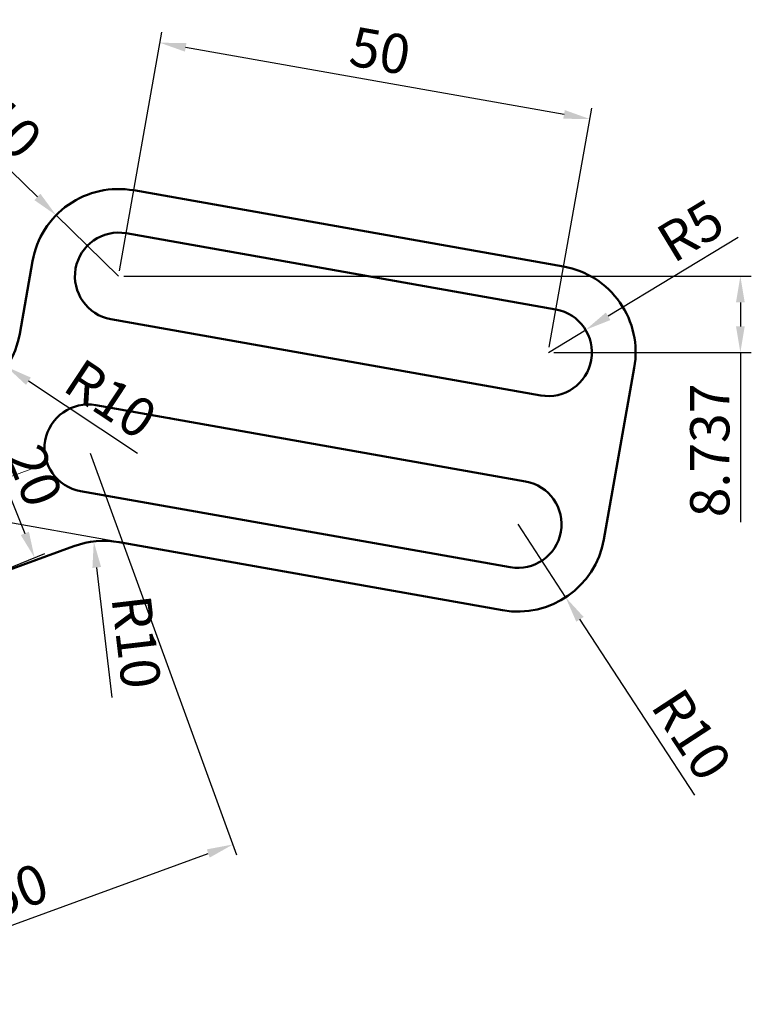
# Model space of a CAD drawing. Units: millimetres. Extents: x 54 to 254, y 16 to 193.
# Tile 2 of 2: x 170 to 254, y 27 to 140. Entities that reach past the tile are written whole.
import ezdxf

# ---------------------------------------------------------------- set-up
doc = ezdxf.new("R2010")
doc.units = ezdxf.units.MM
doc.linetypes.add('CENTER', pattern=[50.8, 31.75, -6.35, 6.35, -6.35])
for name, color, linetype, lineweight in [('M-CNTR', 1, 'CENTER', 18), ('M-DIMS', 2, 'Continuous', 25), ('M-OUTL', 7, 'Continuous', 50)]:
    doc.layers.add(name, color=color, linetype=linetype, lineweight=lineweight)
doc.styles.get("Standard").update_dxf_attribs({"font": 'arial.ttf'})
doc.dimstyles.new('ISO-25', dxfattribs={"dimtxt": 4.5, "dimasz": 3, "dimexe": 1.25, "dimexo": 0.625, "dimtad": 1, "dimdec": 0, "dimtxsty": 'Standard', "dimcen": 2.5, "dimadec": 0, "dimazin": 0, "dimtfac": 1, "dimtdec": 0, "dimtmove": 0, "dimatfit": 3, "dimfxl": 1, "dimarcsym": 0})

# ---------------------------------------------------------------- blocks, each defined once
blk = doc.blocks.new('*D2')
at = {"layer": 'Defpoints', "color": 0, "transparency": 16777216}
for p in [(186.4, 137.25), (181.65, 110.49), (230.91, 101.75)]:
    blk.add_point(p, dxfattribs=at)
at = {"layer": 'M-DIMS', "color": 0, "lineweight": -2, "transparency": 16777216}
for p, q in [((181.76, 111.11), (186.62, 138.48)), ((232.7, 129.04), (189.35, 136.72)), ((231.01, 102.37), (235.87, 129.74))]:
    blk.add_line(p, q, dxfattribs=at)
at = {"layer": 'M-DIMS', "color": 0, "transparency": 16777216}
for points in [[(189.44, 137.22), (189.27, 136.23), (186.4, 137.25)], [(232.79, 129.53), (232.61, 128.54), (235.65, 128.51)]]:
    blk.add_solid(points, dxfattribs=at)
at = {"layer": 'M-DIMS', "color": 0, "transparency": 16777216, "insert": (211.54, 135.76), "char_height": 4.5, "attachment_point": 5, "rotation": 349.9405}
blk.add_mtext('50', dxfattribs=at)
blk = doc.blocks.new('*D20')
at = {"layer": 'Defpoints', "color": 0, "transparency": 16777216}
for p in [(155.74, 93.25), (172.04, 78.24), (163.21, 74.69)]:
    blk.add_point(p, dxfattribs=at)
at = {"layer": 'M-DIMS', "color": 0, "lineweight": -2, "transparency": 16777216}
for p, q in [((156.32, 93.48), (165.74, 97.27)), ((165.7, 94.02), (170.92, 81.02)), ((163.79, 74.92), (173.2, 78.7))]:
    blk.add_line(p, q, dxfattribs=at)
at = {"layer": 'M-DIMS', "color": 0, "transparency": 16777216}
for points in [[(166.16, 94.21), (165.23, 93.83), (164.58, 96.8)], [(171.39, 81.21), (170.46, 80.83), (172.04, 78.24)]]:
    blk.add_solid(points, dxfattribs=at)
at = {"layer": 'M-DIMS', "color": 0, "transparency": 16777216, "insert": (171.5, 87.42), "char_height": 4.5, "attachment_point": 5, "rotation": 291.9033}
blk.add_mtext('20', dxfattribs=at)
blk = doc.blocks.new('*D23')
at = {"layer": 'Defpoints', "color": 0, "transparency": 16777216}
for p in [(178.82, 80.09), (179.98, 70.16)]:
    blk.add_point(p, dxfattribs=at)
at = {"layer": 'M-DIMS', "color": 0, "lineweight": -2, "transparency": 16777216}
blk.add_line((180.92, 62.23), (179.17, 77.11), dxfattribs=at)
at = {"layer": 'M-DIMS', "color": 0, "transparency": 16777216}
blk.add_solid([(179.66, 77.17), (178.67, 77.06), (178.82, 80.09)], dxfattribs=at)
at = {"layer": 'M-DIMS', "color": 0, "transparency": 16777216, "insert": (183.12, 68.52), "char_height": 4.5, "attachment_point": 5, "rotation": 276.7092}
blk.add_mtext('R10', dxfattribs=at)
blk = doc.blocks.new('*D24')
at = {"layer": 'Defpoints', "color": 0, "transparency": 16777216}
for p in [(178.18, 90.79), (131.21, 73.65), (194.76, 45.37)]:
    blk.add_point(p, dxfattribs=at)
at = {"layer": 'M-DIMS', "color": 0, "lineweight": -2, "transparency": 16777216}
for p, q in [((178.4, 90.21), (195.19, 44.19)), ((131.42, 73.07), (148.22, 27.05)), ((150.61, 29.26), (191.94, 44.34))]:
    blk.add_line(p, q, dxfattribs=at)
at = {"layer": 'M-DIMS', "color": 0, "transparency": 16777216}
for points in [[(191.77, 44.81), (192.11, 43.87), (194.76, 45.37)], [(150.43, 29.73), (150.78, 28.79), (147.79, 28.23)]]:
    blk.add_solid(points, dxfattribs=at)
at = {"layer": 'M-DIMS', "color": 0, "transparency": 16777216, "insert": (170.27, 39.54), "char_height": 4.5, "attachment_point": 5, "rotation": 20.0485}
blk.add_mtext('50', dxfattribs=at)
blk = doc.blocks.new('*D25')
at = {"layer": 'Defpoints', "color": 0, "transparency": 16777216}
for p in [(227.41, 82.06), (232.88, 73.69)]:
    blk.add_point(p, dxfattribs=at)
at = {"layer": 'M-DIMS', "color": 0, "lineweight": -2, "transparency": 16777216}
for p, q in [((227.41, 82.06), (232.88, 73.69)), ((247.67, 51.04), (234.52, 71.18))]:
    blk.add_line(p, q, dxfattribs=at)
at = {"layer": 'M-DIMS', "color": 0, "transparency": 16777216}
blk.add_solid([(234.94, 71.45), (234.1, 70.9), (232.88, 73.69)], dxfattribs=at)
at = {"layer": 'M-DIMS', "color": 0, "transparency": 16777216, "insert": (246.84, 57.65), "char_height": 4.5, "attachment_point": 5, "rotation": 303.1406}
blk.add_mtext('R10', dxfattribs=at)
blk = doc.blocks.new('*D26')
at = {"layer": 'Defpoints', "color": 0, "transparency": 16777216}
for p in [(235.18, 104.35), (230.91, 101.75)]:
    blk.add_point(p, dxfattribs=at)
at = {"layer": 'M-DIMS', "color": 0, "lineweight": -2, "transparency": 16777216}
for p, q in [((252.65, 114.94), (237.75, 105.9)), ((230.91, 101.75), (235.18, 104.35))]:
    blk.add_line(p, q, dxfattribs=at)
at = {"layer": 'M-DIMS', "color": 0, "transparency": 16777216}
blk.add_solid([(237.49, 106.33), (238.01, 105.47), (235.18, 104.35)], dxfattribs=at)
at = {"layer": 'M-DIMS', "color": 0, "transparency": 16777216, "insert": (247.49, 115.22), "char_height": 4.5, "attachment_point": 5, "rotation": 31.2309}
blk.add_mtext('R5', dxfattribs=at)
blk = doc.blocks.new('*D27')
at = {"layer": 'Defpoints', "color": 0, "transparency": 16777216}
for p in [(178.18, 90.79), (181.73, 80.01), (156.21, 75.03), (131.21, 73.65), (225.67, 72.21)]:
    blk.add_point(p, dxfattribs=at)
at = {"layer": 'M-DIMS', "color": 0, "lineweight": -2, "transparency": 16777216}
blk.add_line((181.12, 80.12), (167.58, 82.52), dxfattribs=at)
blk.add_arc((159.45, 83.96), 9.5, 218.2164, 331.7726, dxfattribs=at)
at = {"layer": 'M-DIMS', "color": 0, "transparency": 16777216}
for points in [[(167.35, 79.63), (168.3, 79.3), (168.81, 82.3)], [(151.55, 77.84), (152.43, 78.33), (150.53, 80.7)]]:
    blk.add_solid(points, dxfattribs=at)
at = {"layer": 'M-DIMS', "color": 0, "transparency": 16777216, "insert": (160.03, 77.41), "char_height": 4.5, "attachment_point": 5, "rotation": 4.9945}
blk.add_mtext('150°', dxfattribs=at)
blk = doc.blocks.new('SLOT-50X10')
for p, q in [((5.87, 18.66), (55.1, 9.92)), ((4.13, 8.81), (53.36, 0.08))]:
    blk.add_line(p, q)
for centre, start, end in [((5, 13.73), 79.9405, 259.9405), ((54.23, 5), 259.9405, 79.9405)]:
    blk.add_arc(centre, 5, start, end)
blk = doc.blocks.new('*D32')
at = {"layer": 'Defpoints', "color": 0, "transparency": 16777216}
for p in [(181.65, 110.49), (230.91, 101.75), (252.9, 101.75)]:
    blk.add_point(p, dxfattribs=at)
at = {"layer": 'M-DIMS', "color": 0, "lineweight": -2, "transparency": 16777216}
for p, q in [((182.28, 110.49), (254.15, 110.49)), ((252.9, 107.49), (252.9, 104.75)), ((231.53, 101.75), (254.15, 101.75)), ((252.9, 101.75), (252.9, 82.31))]:
    blk.add_line(p, q, dxfattribs=at)
at = {"layer": 'M-DIMS', "color": 0, "transparency": 16777216}
for points in [[(252.4, 107.49), (253.4, 107.49), (252.9, 110.49)], [(252.4, 104.75), (253.4, 104.75), (252.9, 101.75)]]:
    blk.add_solid(points, dxfattribs=at)
at = {"layer": 'M-DIMS', "color": 0, "transparency": 16777216, "insert": (249.98, 90.53), "char_height": 4.5, "attachment_point": 5, "rotation": 90}
blk.add_mtext('8.737', dxfattribs=at)
blk = doc.blocks.new('*D41')
at = {"layer": 'Defpoints', "color": 0, "transparency": 16777216}
for p in [(160.49, 105.63), (168.83, 100.11)]:
    blk.add_point(p, dxfattribs=at)
at = {"layer": 'M-DIMS', "color": 0, "lineweight": -2, "transparency": 16777216}
for p, q in [((160.49, 105.63), (168.83, 100.11)), ((183.83, 90.19), (171.33, 98.46))]:
    blk.add_line(p, q, dxfattribs=at)
at = {"layer": 'M-DIMS', "color": 0, "transparency": 16777216}
blk.add_solid([(171.61, 98.88), (171.06, 98.04), (168.83, 100.11)], dxfattribs=at)
at = {"layer": 'M-DIMS', "color": 0, "transparency": 16777216, "insert": (180.45, 95.94), "char_height": 4.5, "attachment_point": 5, "rotation": 326.5309}
blk.add_mtext('R10', dxfattribs=at)
blk = doc.blocks.new('*D46')
at = {"layer": 'Defpoints', "color": 0, "transparency": 16777216}
for p in [(174.51, 117.48), (181.65, 110.49)]:
    blk.add_point(p, dxfattribs=at)
at = {"layer": 'M-DIMS', "color": 0, "lineweight": -2, "transparency": 16777216}
for p, q in [((154.72, 136.84), (172.36, 119.58)), ((181.65, 110.49), (174.51, 117.48))]:
    blk.add_line(p, q, dxfattribs=at)
at = {"layer": 'M-DIMS', "color": 0, "transparency": 16777216}
blk.add_solid([(172.71, 119.94), (172.01, 119.22), (174.51, 117.48)], dxfattribs=at)
at = {"layer": 'M-DIMS', "color": 0, "transparency": 16777216, "insert": (164.51, 131.35), "char_height": 4.5, "attachment_point": 5, "rotation": 315.6289}
blk.add_mtext('6X R10', dxfattribs=at)

msp = doc.modelspace()

# ---------------------------------------------------------------- linework, layer by layer
at = {"layer": 'M-CNTR'}
msp.add_line((131.2107, 73.6538), (178.1808, 90.7945), dxfattribs=at)
at = {"layer": 'M-OUTL'}
for p, q in [((183.4005, 120.337), (232.6523, 111.5998)), ((170.3358, 103.891), (171.8057, 112.2272)), ((240.7519, 100.0068), (237.2585, 80.3143)), ((187.5455, 94.2113), (187.5751, 94.2221)), ((155.6445, 71.9251), (176.5568, 79.5563)), ((181.7315, 80.0085), (225.6655, 72.2147))]:
    msp.add_line(p, q, dxfattribs=at)
for centre, start, end in [((181.6538, 110.4907), 79.940526, 170), ((230.9056, 101.7535), 349.940514, 79.940526), ((160.4878, 105.6275), 290.047893, 350), ((178.1808, 90.7945), 19.940514, 20.045001), ((179.9848, 70.1622), 79.940514, 110.047893), ((227.4122, 82.061), 259.940514, 349.940514)]:
    msp.add_arc(centre, 10, start, end, dxfattribs=at)

# ---------------------------------------------------------------- block references
at = {"layer": 'M-OUTL', "rotation": 179.99543833143}
msp.add_blockref('SLOT-50X10', (235.896, 115.4855), dxfattribs=at)
at = {"layer": 'M-OUTL'}
msp.add_blockref('SLOT-50X10', (173.181, 77.062), dxfattribs=at)

# ---------------------------------------------------------------- dimensions: what is measured, and where the dimension line sits
at = {"layer": 'M-DIMS'}
dim = msp.add_radius_dim(center=(181.6538, 110.4907), mpoint=(174.5056, 117.4837), text='6X <>', dimstyle='ISO-25', override={"dimdec": 0, "dimlfac": 1, "dimrnd": 0, "dimzin": 0, "dimdsep": 46, "dimlunit": 2}, dxfattribs=at)
dim.commit()
dim.dimension.update_dxf_attribs({"geometry": '*D46', "text_midpoint": (164.5113, 131.3495)})
for p1, p2, distance, picture, middle in [((230.9056, 101.7535), (181.6538, 110.4907), -27.1755, '*D2', (211.5369, 135.7575)), ((131.2107, 73.6538), (178.1808, 90.7945), -48.356, '*D24', (170.271, 39.5439))]:
    dim = msp.add_aligned_dim(p1=p1, p2=p2, distance=distance, dimstyle='ISO-25', override={"dimclrd": 0, "dimclre": 0, "dimclrt": 0}, dxfattribs=at)
    dim.commit()
    dim.dimension.update_dxf_attribs({"geometry": picture, "text_midpoint": middle})
for center, mpoint, picture, middle in [((230.9056, 101.7535), (235.181, 104.346), '*D26', (248.9986, 112.7244)), ((227.4122, 82.061), (232.8791, 73.6877), '*D25', (244.392, 56.0543)), ((179.9848, 70.1622), (178.8165, 80.0938), '*D23', (180.2177, 68.1822))]:
    dim = msp.add_radius_dim(center=center, mpoint=mpoint, dimstyle='ISO-25', override={"dimclrd": 0, "dimclre": 0, "dimclrt": 0}, dxfattribs=at)
    dim.commit()
    dim.dimension.update_dxf_attribs({"geometry": picture, "text_midpoint": middle, "dimtype": 164})
dim = msp.add_linear_dim(base=(252.9033, 101.7535), p1=(181.6538, 110.4907), p2=(230.9056, 101.7535), angle=90, dimstyle='ISO-25', override={"dimdec": 3, "dimlfac": 1, "dimrnd": 0, "dimzin": 0, "dimdsep": 46, "dimlunit": 2}, dxfattribs=at)
dim.commit()
dim.dimension.update_dxf_attribs({"geometry": '*D32', "text_midpoint": (249.9792, 90.5329)})
dim = msp.add_radius_dim(center=(160.4878, 105.6275), mpoint=(168.8296, 100.1127), dimstyle='ISO-25', override={"dimdec": 0, "dimlfac": 1, "dimrnd": 0, "dimzin": 0, "dimdsep": 46, "dimlunit": 2}, dxfattribs=at)
dim.commit()
dim.dimension.update_dxf_attribs({"geometry": '*D41', "text_midpoint": (180.4463, 95.9362)})
dim = msp.add_linear_dim(base=(172.0408, 78.2365), p1=(155.743, 93.2511), p2=(163.2077, 74.685), angle=291.903317, dimstyle='ISO-25', override={"dimclrd": 0, "dimclre": 0, "dimclrt": 0}, dxfattribs=at)
dim.commit()
dim.dimension.update_dxf_attribs({"geometry": '*D20', "text_midpoint": (168.788, 86.3269), "dimtype": 161})
dim = msp.add_angular_dim_2l(base=(156.2064, 75.032), line1=((181.7315, 80.0085), (225.6655, 72.2147)), line2=((131.2107, 73.6538), (178.1808, 90.7945)), dimstyle='ISO-25', override={"dimclrd": 0, "dimclre": 0, "dimclrt": 0}, dxfattribs=at)
dim.commit()
dim.dimension.update_dxf_attribs({"geometry": '*D27', "text_midpoint": (160.0266, 77.4073)})

doc.saveas('drawing.dxf')
